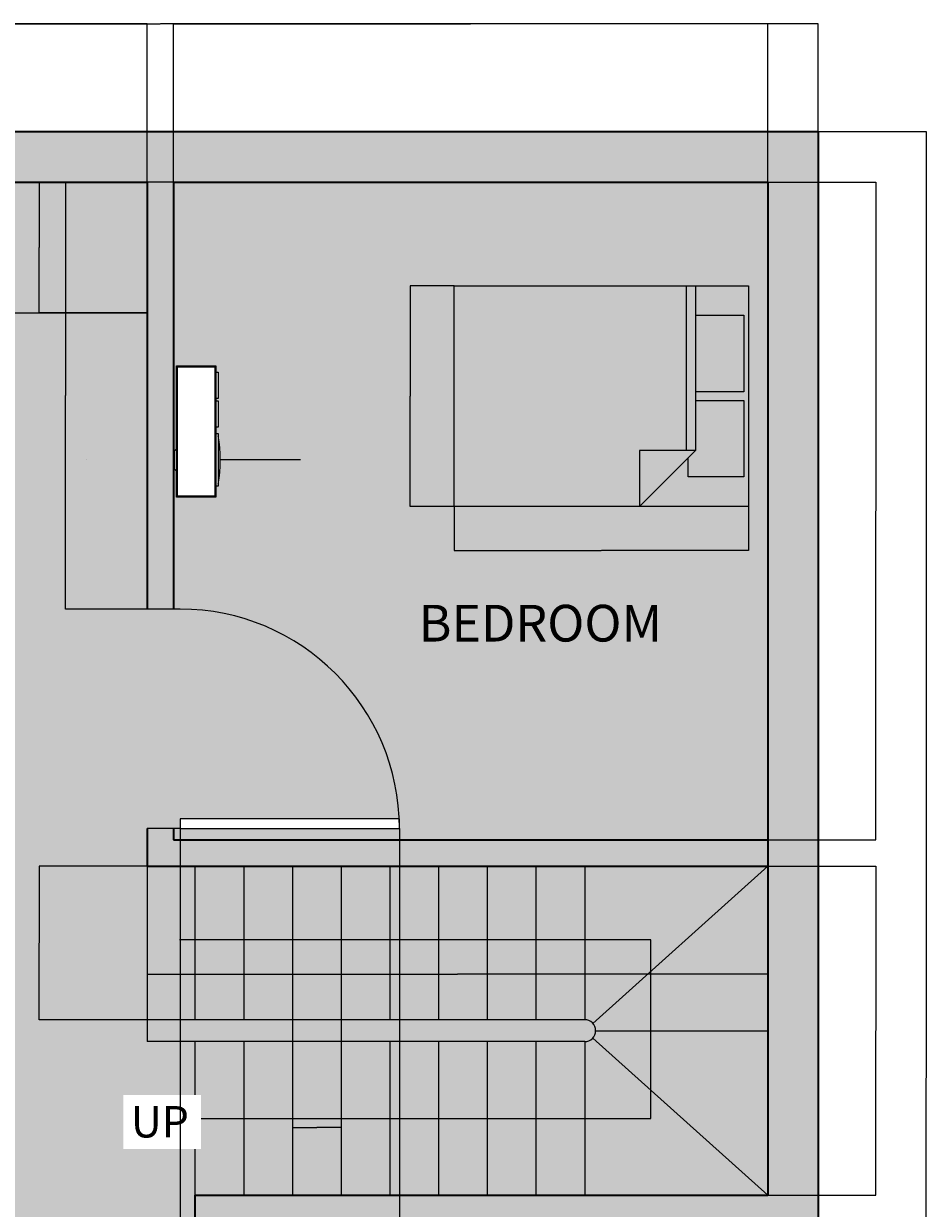
# Model space of a CAD drawing. Units: millimetres. Extents: x 1166 to 16630, y -7192 to 2820.
# Tile 6 of 8: x 4103 to 8218, y -2583 to 2820. Entities that reach past the tile are written whole.
import ezdxf

# ---------------------------------------------------------------- set-up
doc = ezdxf.new("R2010")
doc.units = ezdxf.units.MM
for name, color, linetype, lineweight in [('A-ANNO-DIMS', 2, 'Continuous', 18), ('A-ANNO-SYMB', 7, 'Continuous', 18), ('A-AREA-IDEN', 7, 'Continuous', 18), ('A-DOOR', 4, 'Continuous', 25), ('A-FLOR-CASE', 8, 'Continuous', 18), ('A-FLOR-STRS', 7, 'Continuous', 18), ('A-FURN', 8, 'Continuous', 18), ('A-WALL', 7, 'Continuous', 35)]:
    doc.layers.add(name, color=color, linetype=linetype, lineweight=lineweight)
for name, color, linetype, lineweight, true_color in [('A-FLOR-CASE-PATT', 9, 'Continuous', 13, 0xc7c8ca), ('A-FLOR-FNSH-PATT', 254, 'Continuous', 13, 0xfeeab9), ('A-FURN-PATT', 254, 'Continuous', 13, 0xd7c8d7), ('A-WALL-PATT', 254, 'Continuous', 13, 0xcecce6)]:
    doc.layers.add(name, color=color, linetype=linetype, lineweight=lineweight, true_color=true_color)
doc.styles.get("Standard").update_dxf_attribs({"font": 'arial.ttf'})
doc.dimstyles.get("Standard").update_dxf_attribs({"dimtxt": 0.18, "dimasz": 0.18, "dimexe": 0.18, "dimexo": 0.0625, "dimgap": 0.09, "dimtad": 0, "dimtih": 1, "dimtoh": 1, "dimdec": 4, "dimzin": 0, "dimdsep": 46, "dimtxsty": 'Standard', "dimcen": 0.09, "dimadec": 0, "dimazin": 0, "dimtfac": 1, "dimtdec": 4, "dimtofl": 0, "dimtmove": 0, "dimatfit": 3, "dimfxl": 1, "dimtolj": 1, "dimtzin": 0, "dimarcsym": 0})

# ---------------------------------------------------------------- blocks, each defined once
blk = doc.blocks.new('*U2')
for p, q in [((0, 0), (0, 6)), ((40, 0), (40, 6))]:
    blk.add_line(p, q)
blk.add_lwpolyline([(0, 0), (0, -40), (1.75, -40), (1.75, 0)], close=True)
blk.add_arc((0, 0), 40, 270, 0)
blk = doc.blocks.new('Bed - Queen')
for p, q in [((0, -80.00003), (0, 0)), ((0, 0), (59.99999, 0)), ((59.99999, 0), (59.99999, -80.00003)), ((7.99999, -1.2), (28.79998, -1.2)), ((7.99999, -14.4), (7.99999, -1.2)), ((28.79998, -1.2), (28.79998, -14.4)), ((31.19999, -1.2), (51.99999, -1.2)), ((31.19999, -14.4), (31.19999, -1.2)), ((51.99999, -1.2), (51.99999, -16.4)), ((0, -14.4), (44.8, -14.4)), ((59.99999, -29.6), (44.8, -14.4)), ((44.8, -14.4), (44.8, -29.6)), ((44.8, -16.8), (0, -16.8)), ((51.99999, -16.4), (46.79936, -16.4)), ((44.8, -29.6), (59.99999, -29.6)), ((59.99999, -80.00003), (0, -80.00003))]:
    blk.add_line(p, q)
blk = doc.blocks.new('Entertainment Center')
for p, q in [((-4, 0), (-5, -1)), ((4, 0), (-4, 0)), ((5, -1), (4, 0)), ((-17, -19), (-17, -1)), ((-17, -1), (43, -1)), ((-16.5, -18.5), (-16.5, -1.5)), ((-16.5, -1.5), (42.5, -1.5)), ((42.5, -1.5), (42.5, -18.5)), ((43, -1), (43, -19)), ((43, -19), (-17, -19)), ((42.5, -18.5), (-16.5, -18.5)), ((-12, -20), (-12, -19)), ((12, -20), (-12, -20)), ((12, -19), (12, -20)), ((15, -20), (15, -19)), ((27, -20), (15, -20)), ((27, -19), (27, -20)), ((28, -20), (28, -19)), ((40, -20), (28, -20)), ((40, -19), (40, -20))]:
    blk.add_line(p, q)
blk.add_arc((0, 40), 61, 259.6111, 280.3889)
blk = doc.blocks.new('*D13')
at = {"layer": 'A-ANNO-DIMS', "color": 0, "lineweight": -2, "transparency": 16777216}
for p, q in [((6066.1, 618.4), (6066.1, 417.1)), ((7407.1, 618.4), (7407.1, 417.1)), ((6066.3, 417.3), (6735.5, 417.3)), ((7406.9, 417.3), (6737.7, 417.3))]:
    blk.add_line(p, q, dxfattribs=at)
at = {"layer": 'A-ANNO-DIMS', "color": 0, "transparency": 16777216}
for points in [[(6066.3, 417.3), (6066.3, 417.2), (6066.1, 417.3)], [(7406.9, 417.3), (7406.9, 417.2), (7407.1, 417.3)]]:
    blk.add_solid(points, dxfattribs=at)
at = {"layer": 'Defpoints', "color": 0, "transparency": 16777216}
for p in [(6066.1, 618.4), (7407.1, 618.4), (7407.1, 417.3)]:
    blk.add_point(p, dxfattribs=at)
at = {"layer": 'A-ANNO-DIMS', "color": 0, "transparency": 16777216, "insert": (6736.6, 417.3), "char_height": 0.18, "attachment_point": 5}
blk.add_mtext('\\A1;QUEEN BED 1341', dxfattribs=at)
blk = doc.blocks.new('*D14')
at = {"layer": 'A-ANNO-DIMS', "color": 0, "lineweight": -2, "transparency": 16777216}
for p, q in [((6066, 1624.2), (5864.7, 1624.2)), ((5864.9, 1624), (5864.9, 1121.5)), ((5864.9, 618.6), (5864.9, 1121.1)), ((6066, 618.4), (5864.7, 618.4))]:
    blk.add_line(p, q, dxfattribs=at)
at = {"layer": 'A-ANNO-DIMS', "color": 0, "transparency": 16777216}
for points in [[(5864.9, 1624), (5865, 1624), (5864.9, 1624.2)], [(5864.9, 618.6), (5865, 618.6), (5864.9, 618.4)]]:
    blk.add_solid(points, dxfattribs=at)
at = {"layer": 'Defpoints', "color": 0, "transparency": 16777216}
for p in [(6066.1, 1624.2), (5864.9, 618.4), (6066.1, 618.4)]:
    blk.add_point(p, dxfattribs=at)
at = {"layer": 'A-ANNO-DIMS', "color": 0, "transparency": 16777216, "insert": (5864.9, 1121.3), "char_height": 0.18, "attachment_point": 5}
blk.add_mtext('\\A1;1006', dxfattribs=at)
blk = doc.blocks.new('*D23')
at = {"layer": 'A-ANNO-DIMS', "color": 0, "lineweight": -2, "transparency": 16777216}
for p, q in [((1725.9, 2327.5), (1725.9, 2819.6)), ((1726.1, 2819.5), (4725.6, 2819.5)), ((7725.8, 2819.5), (4726.3, 2819.5)), ((7725.9, 2327.5), (7725.9, 2819.6))]:
    blk.add_line(p, q, dxfattribs=at)
at = {"layer": 'A-ANNO-DIMS', "color": 0, "transparency": 16777216}
for points in [[(1726.1, 2819.5), (1726.1, 2819.4), (1725.9, 2819.5)], [(7725.8, 2819.5), (7725.8, 2819.4), (7725.9, 2819.5)]]:
    blk.add_solid(points, dxfattribs=at)
at = {"layer": 'Defpoints', "color": 0, "transparency": 16777216}
for p in [(7725.9, 2819.5), (1725.9, 2327.5), (7725.9, 2327.5)]:
    blk.add_point(p, dxfattribs=at)
at = {"layer": 'A-ANNO-DIMS', "color": 0, "transparency": 16777216, "insert": (4725.9, 2819.5), "char_height": 0.18, "attachment_point": 5}
blk.add_mtext('\\A1;6000', dxfattribs=at)
blk = doc.blocks.new('*D24')
at = {"layer": 'A-ANNO-DIMS', "color": 0, "lineweight": -2, "transparency": 16777216}
for p, q in [((7726, 2327.5), (8218.1, 2327.5)), ((8217.9, 2327.3), (8217.9, -1988.2)), ((8217.9, -6304), (8217.9, -1988.5)), ((7726, -6304.1), (8218.1, -6304.1))]:
    blk.add_line(p, q, dxfattribs=at)
at = {"layer": 'A-ANNO-DIMS', "color": 0, "transparency": 16777216}
for points in [[(8217.9, 2327.3), (8218, 2327.3), (8217.9, 2327.5)], [(8217.9, -6304), (8218, -6304), (8217.9, -6304.1)]]:
    blk.add_solid(points, dxfattribs=at)
at = {"layer": 'Defpoints', "color": 0, "transparency": 16777216}
for p in [(7725.9, 2327.5), (7725.9, -6304.1), (8217.9, -6304.1)]:
    blk.add_point(p, dxfattribs=at)
at = {"layer": 'A-ANNO-DIMS', "color": 0, "transparency": 16777216, "insert": (8217.9, -1988.3), "char_height": 0.18, "attachment_point": 5}
blk.add_mtext('\\A1;8632', dxfattribs=at)
blk = doc.blocks.new('*D25')
at = {"layer": 'A-ANNO-DIMS', "color": 0, "lineweight": -2, "transparency": 16777216}
for p, q in [((1955.939441, 2097.524735), (1955.939441, 2819.642235)), ((1956.119441, 2819.462235), (3310.579441, 2819.462235)), ((4665.759441, 2819.462235), (3311.299441, 2819.462235)), ((4665.939441, 2097.524735), (4665.939441, 2819.642235))]:
    blk.add_line(p, q, dxfattribs=at)
at = {"layer": 'A-ANNO-DIMS', "color": 0, "transparency": 16777216}
for points in [[(1956.119441, 2819.492235), (1956.119441, 2819.432235), (1955.939441, 2819.462235)], [(4665.759441, 2819.492235), (4665.759441, 2819.432235), (4665.939441, 2819.462235)]]:
    blk.add_solid(points, dxfattribs=at)
at = {"layer": 'Defpoints', "color": 0, "transparency": 16777216}
for p in [(4665.939441, 2819.462235), (1955.939441, 2097.462235), (4665.939441, 2097.462235)]:
    blk.add_point(p, dxfattribs=at)
at = {"layer": 'A-ANNO-DIMS', "color": 0, "transparency": 16777216, "insert": (3310.939441, 2819.462235), "char_height": 0.18, "attachment_point": 5}
blk.add_mtext('\\A1;2710', dxfattribs=at)
blk = doc.blocks.new('*D26')
at = {"layer": 'A-ANNO-DIMS', "color": 0, "lineweight": -2, "transparency": 16777216}
for p, q in [((4785.939441, 2097.524735), (4785.939441, 2819.642235)), ((4786.119441, 2819.462235), (6140.579441, 2819.462235)), ((7495.759441, 2819.462235), (6141.299441, 2819.462235)), ((7495.939441, 2097.524735), (7495.939441, 2819.642235))]:
    blk.add_line(p, q, dxfattribs=at)
at = {"layer": 'A-ANNO-DIMS', "color": 0, "transparency": 16777216}
for points in [[(4786.119441, 2819.492235), (4786.119441, 2819.432235), (4785.939441, 2819.462235)], [(7495.759441, 2819.492235), (7495.759441, 2819.432235), (7495.939441, 2819.462235)]]:
    blk.add_solid(points, dxfattribs=at)
at = {"layer": 'Defpoints', "color": 0, "transparency": 16777216}
for p in [(7495.939441, 2819.462235), (4785.939441, 2097.462235), (7495.939441, 2097.462235)]:
    blk.add_point(p, dxfattribs=at)
at = {"layer": 'A-ANNO-DIMS', "color": 0, "transparency": 16777216, "insert": (6140.939441, 2819.462235), "char_height": 0.18, "attachment_point": 5}
blk.add_mtext('\\A1;2710', dxfattribs=at)
blk = doc.blocks.new('*D33')
at = {"layer": 'A-ANNO-DIMS', "color": 0, "lineweight": -2, "transparency": 16777216}
for p, q in [((7496, 2097.5), (7988.1, 2097.5)), ((7987.9, 2097.3), (7987.9, 597.6)), ((7987.9, -902.4), (7987.9, 597.3)), ((7496, -902.5), (7988.1, -902.5))]:
    blk.add_line(p, q, dxfattribs=at)
at = {"layer": 'A-ANNO-DIMS', "color": 0, "transparency": 16777216}
for points in [[(7987.9, 2097.3), (7988, 2097.3), (7987.9, 2097.5)], [(7987.9, -902.4), (7988, -902.4), (7987.9, -902.5)]]:
    blk.add_solid(points, dxfattribs=at)
at = {"layer": 'Defpoints', "color": 0, "transparency": 16777216}
for p in [(7495.9, 2097.5), (7495.9, -902.5), (7987.9, -902.5)]:
    blk.add_point(p, dxfattribs=at)
at = {"layer": 'A-ANNO-DIMS', "color": 0, "transparency": 16777216, "insert": (7987.9, 597.5), "char_height": 0.18, "attachment_point": 5}
blk.add_mtext('\\A1;3000', dxfattribs=at)
blk = doc.blocks.new('*D34')
at = {"layer": 'A-ANNO-DIMS', "color": 0, "lineweight": -2, "transparency": 16777216}
for p, q in [((7496, -1022.5), (7988.1, -1022.5)), ((7987.9, -1022.7), (7987.9, -1772.4)), ((7987.9, -2522.4), (7987.9, -1772.7)), ((7496, -2522.5), (7988.1, -2522.5))]:
    blk.add_line(p, q, dxfattribs=at)
at = {"layer": 'A-ANNO-DIMS', "color": 0, "transparency": 16777216}
for points in [[(7987.9, -1022.7), (7988, -1022.7), (7987.9, -1022.5)], [(7987.9, -2522.4), (7988, -2522.4), (7987.9, -2522.5)]]:
    blk.add_solid(points, dxfattribs=at)
at = {"layer": 'Defpoints', "color": 0, "transparency": 16777216}
for p in [(7495.9, -1022.5), (7495.9, -2522.5), (7987.9, -2522.5)]:
    blk.add_point(p, dxfattribs=at)
at = {"layer": 'A-ANNO-DIMS', "color": 0, "transparency": 16777216, "insert": (7987.9, -1772.5), "char_height": 0.18, "attachment_point": 5}
blk.add_mtext('\\A1;1500', dxfattribs=at)
blk = doc.blocks.new('*D36')
at = {"layer": 'A-ANNO-DIMS', "color": 0, "lineweight": -2, "transparency": 16777216}
for p, q in [((4815.9, -849.9), (4815.9, -7065.6)), ((5815.9, -849.9), (5815.9, -7065.6)), ((4816.1, -7065.4), (5315.6, -7065.4)), ((5815.8, -7065.4), (5316.3, -7065.4))]:
    blk.add_line(p, q, dxfattribs=at)
at = {"layer": 'A-ANNO-DIMS', "color": 0, "transparency": 16777216}
for points in [[(4816.1, -7065.4), (4816.1, -7065.5), (4815.9, -7065.4)], [(5815.8, -7065.4), (5815.8, -7065.5), (5815.9, -7065.4)]]:
    blk.add_solid(points, dxfattribs=at)
at = {"layer": 'Defpoints', "color": 0, "transparency": 16777216}
for p in [(4815.9, -849.8), (5815.9, -849.8), (5815.9, -7065.4)]:
    blk.add_point(p, dxfattribs=at)
at = {"layer": 'A-ANNO-DIMS', "color": 0, "transparency": 16777216, "insert": (5315.9, -7065.4), "char_height": 0.18, "attachment_point": 5}
blk.add_mtext('\\A1;1000', dxfattribs=at)
blk = doc.blocks.new('*D40')
at = {"layer": 'A-ANNO-DIMS', "color": 0, "lineweight": -2, "transparency": 16777216}
for p, q in [((4665.9, 2097.5), (4173.8, 2097.5)), ((4173.9, 2097.3), (4173.9, 1799.3)), ((4173.9, 1500.9), (4173.9, 1798.9)), ((4665.9, 1500.7), (4173.8, 1500.7))]:
    blk.add_line(p, q, dxfattribs=at)
at = {"layer": 'A-ANNO-DIMS', "color": 0, "transparency": 16777216}
for points in [[(4173.9, 2097.3), (4174, 2097.3), (4173.9, 2097.5)], [(4173.9, 1500.9), (4174, 1500.9), (4173.9, 1500.7)]]:
    blk.add_solid(points, dxfattribs=at)
at = {"layer": 'Defpoints', "color": 0, "transparency": 16777216}
for p in [(4173.9, 2097.5), (4665.9, 2097.5), (4665.9, 1500.7)]:
    blk.add_point(p, dxfattribs=at)
at = {"layer": 'A-ANNO-DIMS', "color": 0, "transparency": 16777216, "insert": (4173.9, 1799.1), "char_height": 0.18, "attachment_point": 5}
blk.add_mtext('\\A1;596.8', dxfattribs=at)
blk = doc.blocks.new('*D42')
at = {"layer": 'A-ANNO-DIMS', "color": 0, "lineweight": -2, "transparency": 16777216}
for p, q in [((4785.9, 2097.5), (4293.8, 2097.5)), ((4293.9, 2097.3), (4293.9, 1124)), ((4293.9, 150.4), (4293.9, 1123.6)), ((4785.9, 150.2), (4293.8, 150.2))]:
    blk.add_line(p, q, dxfattribs=at)
at = {"layer": 'A-ANNO-DIMS', "color": 0, "transparency": 16777216}
for points in [[(4293.9, 2097.3), (4294, 2097.3), (4293.9, 2097.5)], [(4293.9, 150.4), (4294, 150.4), (4293.9, 150.2)]]:
    blk.add_solid(points, dxfattribs=at)
at = {"layer": 'Defpoints', "color": 0, "transparency": 16777216}
for p in [(4293.9, 2097.5), (4785.9, 2097.5), (4785.9, 150.2)]:
    blk.add_point(p, dxfattribs=at)
at = {"layer": 'A-ANNO-DIMS', "color": 0, "transparency": 16777216, "insert": (4293.9, 1123.8), "char_height": 0.18, "attachment_point": 5}
blk.add_mtext('\\A1;1947.3', dxfattribs=at)
blk = doc.blocks.new('*D44')
at = {"layer": 'A-ANNO-DIMS', "color": 0, "lineweight": -2, "transparency": 16777216}
for p, q in [((4665.9, -1022.5), (4173.8, -1022.5)), ((4173.9, -1022.7), (4173.9, -1372.4)), ((4173.9, -1722.4), (4173.9, -1372.7)), ((4665.9, -1722.5), (4173.8, -1722.5))]:
    blk.add_line(p, q, dxfattribs=at)
at = {"layer": 'A-ANNO-DIMS', "color": 0, "transparency": 16777216}
for points in [[(4173.9, -1022.7), (4174, -1022.7), (4173.9, -1022.5)], [(4173.9, -1722.4), (4174, -1722.4), (4173.9, -1722.5)]]:
    blk.add_solid(points, dxfattribs=at)
at = {"layer": 'Defpoints', "color": 0, "transparency": 16777216}
for p in [(4173.9, -1022.5), (4665.9, -1022.5), (4665.9, -1722.5)]:
    blk.add_point(p, dxfattribs=at)
at = {"layer": 'A-ANNO-DIMS', "color": 0, "transparency": 16777216, "insert": (4173.9, -1372.5), "char_height": 0.18, "attachment_point": 5}
blk.add_mtext('\\A1;700', dxfattribs=at)
blk = doc.blocks.new('*D45')
at = {"layer": 'A-ANNO-DIMS', "color": 0, "lineweight": -2, "transparency": 16777216}
for p, q in [((5328.2, -1722.6), (5328.2, -2214.7)), ((5550.3, -1722.6), (5550.3, -2214.7)), ((5328.4, -2214.5), (5438.9, -2214.5)), ((5550.1, -2214.5), (5439.6, -2214.5))]:
    blk.add_line(p, q, dxfattribs=at)
at = {"layer": 'A-ANNO-DIMS', "color": 0, "transparency": 16777216}
for points in [[(5328.4, -2214.5), (5328.4, -2214.6), (5328.2, -2214.5)], [(5550.1, -2214.5), (5550.1, -2214.6), (5550.3, -2214.5)]]:
    blk.add_solid(points, dxfattribs=at)
at = {"layer": 'Defpoints', "color": 0, "transparency": 16777216}
for p in [(5328.2, -1722.5), (5550.3, -1722.5), (5328.2, -2214.5)]:
    blk.add_point(p, dxfattribs=at)
at = {"layer": 'A-ANNO-DIMS', "color": 0, "transparency": 16777216, "insert": (5439.2, -2214.5), "char_height": 0.18, "attachment_point": 5}
blk.add_mtext('\\A1;222.1', dxfattribs=at)
blk = doc.blocks.new('*D46')
at = {"layer": 'A-ANNO-DIMS', "color": 0, "lineweight": -2, "transparency": 16777216}
for p, q in [((4665.939441, -1022.600265), (4665.939441, -1514.717765)), ((7495.939441, -1022.600265), (7495.939441, -1514.717765)), ((4666.119441, -1514.537765), (6080.579441, -1514.537765)), ((7495.759441, -1514.537765), (6081.299441, -1514.537765))]:
    blk.add_line(p, q, dxfattribs=at)
at = {"layer": 'A-ANNO-DIMS', "color": 0, "transparency": 16777216}
for points in [[(4666.119441, -1514.507765), (4666.119441, -1514.567765), (4665.939441, -1514.537765)], [(7495.759441, -1514.507765), (7495.759441, -1514.567765), (7495.939441, -1514.537765)]]:
    blk.add_solid(points, dxfattribs=at)
at = {"layer": 'Defpoints', "color": 0, "transparency": 16777216}
for p in [(4665.939441, -1022.537765), (7495.939441, -1022.537765), (4665.939441, -1514.537765)]:
    blk.add_point(p, dxfattribs=at)
at = {"layer": 'A-ANNO-DIMS', "color": 0, "transparency": 16777216, "insert": (6080.939441, -1514.537765), "char_height": 0.18, "attachment_point": 5}
blk.add_mtext('\\A1;2830', dxfattribs=at)
blk = doc.blocks.new('*D71')
at = {"layer": 'A-ANNO-DIMS', "color": 0, "lineweight": -2, "transparency": 16777216}
for p, q in [((4389.3, 830.2), (4389.5, 830.2)), ((4389.4, 830.1), (4389.4, 830.2)), ((5365.1, 830.2), (4999.4, 830.2))]:
    blk.add_line(p, q, dxfattribs=at)
at = {"layer": 'A-ANNO-DIMS', "color": 0, "transparency": 16777216}
blk.add_solid([(4999.4, 830.2), (4999.4, 830.1), (4999.2, 830.2)], dxfattribs=at)
at = {"layer": 'Defpoints', "color": 0, "transparency": 16777216}
for p in [(4389.4, 830.2), (4999.2, 830.2)]:
    blk.add_point(p, dxfattribs=at)
at = {"layer": 'A-ANNO-DIMS', "color": 0, "transparency": 16777216, "insert": (5365.5, 830.2), "char_height": 0.18, "attachment_point": 5}
blk.add_mtext('\\A1;R609.8', dxfattribs=at)

msp = doc.modelspace()

# ---------------------------------------------------------------- hatches: boundary and pattern name
at = {"layer": 'A-FLOR-CASE-PATT'}
h = msp.add_hatch(color=256, dxfattribs=at)
h.dxf.hatch_style = 1
h.paths.add_polyline_path([(2460.545, 1500.697), (4665.939, 1500.697), (4665.939, 2097.462), (1955.939, 2097.462), (1955.939, -402.538), (2460.545, -402.538)])
at = {"layer": 'A-FLOR-FNSH-PATT', "transparency": 33554523}
h = msp.add_hatch(color=256, dxfattribs=at)
h.dxf.hatch_style = 1
h.paths.add_polyline_path([(7725.939, 2327.462), (1725.939, 2327.462), (1725.939, -5672.538), (5309.615, -5672.538), (5309.615, -2642.538), (5189.615, -2642.538), (5189.615, -5442.538), (1955.939, -5442.538), (1955.939, 2097.462), (4665.939, 2097.462), (4665.939, 150.2), (4815.939, 150.2, -0.40145271), (5814.982, -806.05), (5815.939, -806.05), (5815.939, -849.8), (4815.939, -849.8), (4785.939, -849.8), (4785.939, -902.538), (7495.939, -902.538), (7495.939, -2522.538), (4884.014, -2522.538), (4884.014, -2642.538), (7725.939, -2642.538)], flags=17)
h.paths.add_polyline_path([(6066.077, 618.421), (6066.077, 1624.186), (7407.098, 1624.186), (7407.098, 618.421)], flags=16)
h.paths.add_polyline_path([(4979.212, 660.219), (4799.278, 660.219), (4799.278, 780.174), (4789.282, 790.171), (4789.282, 870.141), (4799.278, 880.137), (4799.278, 1259.997), (4979.212, 1259.997), (4979.212, 1230.008), (4989.208, 1230.008), (4989.208, 1110.052), (4979.212, 1110.052), (4979.212, 1100.056), (4989.208, 1100.056), (4989.208, 980.1), (4979.212, 980.1), (4979.212, 950.111), (4989.208, 950.111), (4989.208, 940.115, -0.09090909), (4989.208, 720.196), (4989.208, 710.2), (4979.212, 710.2)], flags=16)
h.paths.add_polyline_path([(4974.214, 665.217), (4804.276, 665.217), (4804.276, 1254.999), (4974.214, 1254.999)], flags=0)
h.paths.add_polyline_path([(6910.92, 618.421), (6910.92, 873.215), (7165.714, 873.215), (7165.714, 1490.084), (7386.983, 1490.084), (7386.983, 1141.419), (7165.714, 1141.419), (7165.714, 1101.188), (7386.983, 1101.188), (7386.983, 752.523), (7132.189, 752.523), (7132.189, 839.689)], flags=16)
h.paths.add_polyline_path([(4815.939, 150.2), (4665.939, 150.2), (4665.939, 1500.697), (2460.545, 1500.697), (2460.545, -402.538), (3575.939, -402.538), (3575.939, -1706.64), (3463.439, -1706.64, 0.40145271), (2714.158, -2423.828), (3463.439, -2423.828), (3463.439, -2456.64), (3455.939, -2522.538), (3455.939, -2456.64), (2713.439, -2456.64), (2713.439, -2423.828), (2714.158, -2423.828, -0.39855266), (3455.939, -1706.678), (3455.939, -1706.64), (3575.939, -1706.64), (3575.939, -402.538), (2460.545, -402.538), (2460.545, 1500.697), (4665.939, 1500.697), (4665.939, 150.2), (4785.939, 150.2), (4785.939, 2097.462), (7495.939, 2097.462), (7495.939, -2522.538), (4884.014, -2522.538), (4884.014, -2642.538), (7725.939, -2642.538), (7725.939, 2327.462), (1725.939, 2327.462), (1725.939, -5672.538), (5309.615, -5672.538), (5309.615, -2642.538), (4884.014, -2642.538), (4884.014, -2522.538), (4884.014, -1822.538), (4665.939, -1822.538), (4665.939, -1722.538), (4665.939, -1022.538), (4665.939, -849.8), (4815.939, -849.8), (4815.939, -806.05), (5814.982, -806.05, 0.40145271)])
h.paths.add_polyline_path([(1955.939, -4323.626), (1965.936, -4313.63), (1965.936, -3933.77), (2145.869, -3933.77), (2145.869, -3963.759), (2155.866, -3963.759), (2155.866, -4083.715), (2145.869, -4083.715), (2145.869, -4093.711), (2155.866, -4093.711), (2155.866, -4213.667), (2145.869, -4213.667), (2145.869, -4243.656), (2155.866, -4243.656), (2155.866, -4253.652, -0.09090909), (2155.866, -4473.571), (2155.866, -4483.567), (2145.869, -4483.567), (2145.869, -4533.549), (1965.936, -4533.549), (1965.936, -4413.593), (1955.939, -4403.597)], flags=16)
h.paths.add_polyline_path([(3017.672, -1268.685), (3017.672, -1558.932), (2092.538, -1558.932), (2092.538, -1268.685)], flags=16)
h.paths.add_polyline_path([(2768.799, -687.028), (2664.904, -687.028), (2696.871, -782.93, -0.50132349), (2617.667, -1084.405, -0.13289091), (2584.271, -1084.405, -0.50131678), (2505.065, -782.933), (2537.033, -687.028), (2489.082, -687.028), (2489.082, -711.004), (2441.13, -711.004), (2441.13, -687.028), (2433.138, -687.028), (2433.138, -559.158), (2768.799, -559.158)], flags=16)
h.paths.add_polyline_path([(2752.815, -655.061, -0.41421356), (2740.827, -671.045), (2465.106, -671.045, -0.41421356), (2449.122, -659.057), (2449.122, -591.126, -0.41421356), (2461.11, -575.142), (2736.831, -575.142, -0.41421356), (2752.815, -587.13)], flags=0)
h.paths.add_polyline_path([(2627.247, -1063.016, -0.21500378), (2574.691, -1063.016, -0.48007965), (2537.034, -782.931), (2664.904, -782.931, -0.4800795)], flags=0)
h.paths.add_polyline_path([(4505.634, -3647.875), (4977.863, -3647.875, -0.19047621), (4977.864, -5173.541), (4505.634, -5173.541), (4505.634, -5064.565), (4533.929, -5064.565), (4533.929, -3756.851), (4505.634, -3756.851)], flags=16)
h.paths.add_polyline_path([(4880.114, -4192.756), (5003.372, -4192.756, -0.04962821), (5003.372, -4628.66), (4880.114, -4628.66)], flags=0)
h.paths.add_polyline_path([(2140.871, -3938.769), (2140.871, -4528.551), (1970.934, -4528.551), (1970.934, -3938.769)], flags=0)
h.paths.add_polyline_path([(7495.939, -1022.538), (6660.699, -1022.538), (6660.699, -1722.538, -0.21291191), (6697.901, -1739.132)], flags=16)
h.paths.add_polyline_path([(7495.939, -1022.538), (6697.901, -1739.132, -0.18498743), (6710.699, -1772.538), (7495.939, -1772.538)], flags=16)
h.paths.add_polyline_path([(7495.939, -1772.538), (6710.699, -1772.538, -0.18498743), (6697.901, -1805.944), (7495.939, -2522.538)], flags=16)
h.paths.add_polyline_path([(6697.901, -1805.944, -0.21291191), (6660.699, -1822.538), (6660.699, -2522.538), (7495.939, -2522.538)], flags=16)
h.paths.add_polyline_path([(6660.699, -1822.538), (6438.613, -1822.538), (6438.613, -2522.538), (6660.699, -2522.538)], flags=16)
h.paths.add_polyline_path([(6438.613, -1822.538), (6216.528, -1822.538), (6216.528, -2522.538), (6438.613, -2522.538)], flags=16)
h.paths.add_polyline_path([(6216.528, -1822.538), (5994.442, -1822.538), (5994.442, -2522.538), (6216.528, -2522.538)], flags=16)
h.paths.add_polyline_path([(5994.442, -1822.538), (5772.357, -1822.538), (5772.357, -2522.538), (5994.442, -2522.538)], flags=16)
h.paths.add_polyline_path([(5550.271, -1822.538), (5328.185, -1822.538), (5328.185, -2522.538), (5550.271, -2522.538)], flags=16)
h.paths.add_polyline_path([(5328.185, -1822.538), (5106.1, -1822.538), (5106.1, -2522.538), (5328.185, -2522.538)], flags=16)
h.paths.add_polyline_path([(5106.1, -1822.538), (4884.014, -1822.538), (4884.014, -2522.538), (5106.1, -2522.538)], flags=16)
h.paths.add_polyline_path([(4884.014, -1022.538), (4665.939, -1022.538), (4665.939, -1722.538), (4884.014, -1722.538)], flags=16)
h.paths.add_polyline_path([(5106.1, -1022.538), (4884.014, -1022.538), (4884.014, -1722.538), (5106.1, -1722.538)], flags=16)
h.paths.add_polyline_path([(5550.271, -1022.538), (5328.185, -1022.538), (5328.185, -1722.538), (5550.271, -1722.538)], flags=16)
h.paths.add_polyline_path([(5328.185, -1022.538), (5106.1, -1022.538), (5106.1, -1722.538), (5328.185, -1722.538)], flags=16)
h.paths.add_polyline_path([(5772.357, -1022.538), (5550.271, -1022.538), (5550.271, -1722.538), (5772.357, -1722.538)], flags=16)
h.paths.add_polyline_path([(5994.442, -1022.538), (5772.357, -1022.538), (5772.357, -1722.538), (5994.442, -1722.538)], flags=16)
h.paths.add_polyline_path([(6216.528, -1022.538), (5994.442, -1022.538), (5994.442, -1722.538), (6216.528, -1722.538)], flags=16)
h.paths.add_polyline_path([(6660.699, -1022.538), (6438.613, -1022.538), (6438.613, -1722.538), (6660.699, -1722.538)], flags=16)
h.paths.add_polyline_path([(6438.613, -1022.538), (6216.528, -1022.538), (6216.528, -1722.538), (6438.613, -1722.538)], flags=16)
h.paths.add_polyline_path([(5772.357, -1822.538), (5550.271, -1822.538), (5550.271, -2522.538), (5772.357, -2522.538)], flags=16)
h.paths.add_polyline_path([(6660.699, -1722.538), (6438.613, -1722.538), (4665.939, -1722.538), (4665.939, -1822.538), (6660.699, -1822.538, 0.21291191), (6697.901, -1805.944, 0.64892437)], flags=16)
h.paths.add_polyline_path([(5860.25, -44.006), (7154.504, -44.006), (7154.504, 215.689), (5860.25, 215.689)], flags=24)
h.paths.add_polyline_path([(2102.336, -1543.656), (3007.075, -1543.656), (3007.075, -1283.961), (2102.336, -1283.961)], flags=8)
h.paths.add_polyline_path([(2887.503, -4248.68), (3740.372, -4248.68), (3740.372, -3989.156), (2887.503, -3989.156)], flags=24)
h.paths.add_polyline_path([(2999.436, 433.054), (4111.829, 433.054), (4111.829, 692.578), (2999.436, 692.578)], flags=24)
at = {"layer": 'A-FLOR-FNSH-PATT', "transparency": 33554590}
h = msp.add_hatch(color=256, dxfattribs=at)
h.dxf.hatch_style = 1
h.paths.add_polyline_path([(5309.615, -2642.538), (5309.615, -6304.141), (7725.939, -6304.141), (7725.939, -5672.538), (7725.939, -2642.538)])
edge = h.paths.add_edge_path(flags=16)
edge.add_ellipse((-448.972, -3645.43), major_axis=(-7430.723, 0), ratio=0.84230387, start_angle=182.1799503, end_angle=183.6504276, ccw=False)
edge.add_line((6974.174, -3362.862), (6984.716, -3362.862))
edge.add_ellipse((6982.281, -3380.397), major_axis=(-20.817, 0), ratio=0.84230387, start_angle=180, end_angle=270, ccw=False)
edge.add_line((7003.098, -3380.397), (7003.098, -3722.916))
edge.add_ellipse((6982.281, -3720.865), major_axis=(20.817, 0), ratio=0.84230387, start_angle=270, end_angle=360, ccw=False)
edge.add_ellipse((-142030.923, -3973.064), major_axis=(149013.204, 0), ratio=0.8423038695, start_angle=-0.38386678, end_angle=0.09022909, ccw=False)
edge.add_line((6977.567, -4971.397), (6984.47, -4971.397))
edge.add_ellipse((6982.281, -4988.932), major_axis=(20.817, 0), ratio=0.84230387, start_angle=0, end_angle=90, ccw=False)
edge.add_line((7003.098, -4988.932), (7003.098, -5331.243))
edge.add_ellipse((6982.281, -5329.4), major_axis=(-20.817, 0), ratio=0.84230387, start_angle=90, end_angle=180, ccw=False)
edge.add_line((6982.281, -5346.934), (6973.354, -5346.934))
edge.add_ellipse((-142030.923, -3973.064), major_axis=(149013.204, 0), ratio=0.8423038695, start_angle=-0.6186432, end_angle=-0.52827147, ccw=False)
edge.add_ellipse((6960.189, -5606.903), major_axis=(-31.226, 0), ratio=0.84230387, start_angle=179.371763, end_angle=248.464757, ccw=False)
edge.add_ellipse((-142041.332, -3973.064), major_axis=(-149045.372, 0), ratio=0.8423038661, start_angle=179.35344592, end_angle=179.3717628, ccw=False)
edge.add_ellipse((6916.87, -5654.054), major_axis=(-73.802, 0), ratio=0.84230387, start_angle=90, end_angle=179.353446, ccw=False)
edge.add_line((6916.87, -5716.218), (5995.23, -5716.218))
edge.add_ellipse((5995.23, -5654.054), major_axis=(73.802, 0), ratio=0.84230387, start_angle=180.646554, end_angle=270, ccw=False)
edge.add_ellipse((154953.432, -3973.064), major_axis=(-149045.372, 0), ratio=0.8423038697, start_angle=0.62823722, end_angle=0.6465541, ccw=False)
edge.add_ellipse((5951.911, -5606.903), major_axis=(31.226, 0), ratio=0.84230387, start_angle=111.535244, end_angle=180.628237, ccw=False)
edge.add_ellipse((154943.023, -3973.064), major_axis=(-149013.204, 0), ratio=0.8423038695, start_angle=0.52827147, end_angle=0.6465541, ccw=False)
edge.add_line((5938.746, -5346.934), (5927.384, -5346.934))
edge.add_ellipse((5929.819, -5329.4), major_axis=(20.817, 0), ratio=0.84230387, start_angle=180, end_angle=270, ccw=False)
edge.add_line((5909.002, -5329.4), (5909.002, -4986.881))
edge.add_ellipse((5929.819, -4988.932), major_axis=(-20.817, 0), ratio=0.84230387, start_angle=-90, end_angle=0, ccw=False)
edge.add_line((5929.819, -4971.397), (5934.533, -4971.397))
edge.add_ellipse((154943.023, -3973.064), major_axis=(-149013.204, 0), ratio=0.8423038695, start_angle=-0.09022909, end_angle=0.38386678, ccw=False)
edge.add_ellipse((5929.819, -3720.865), major_axis=(-20.817, 0), ratio=0.84230387, start_angle=0, end_angle=90, ccw=False)
edge.add_line((5909.002, -3720.865), (5909.002, -3378.346))
edge.add_ellipse((5929.819, -3380.397), major_axis=(20.817, 0), ratio=0.84230387, start_angle=90, end_angle=180, ccw=False)
edge.add_line((5929.819, -3362.862), (5937.926, -3362.862))
edge.add_ellipse((13361.072, -3645.43), major_axis=(7430.723, 0), ratio=0.84230387, start_angle=176.3495724, end_angle=177.8200497, ccw=False)
edge.add_ellipse((6843.239, -6808.261), major_axis=(4407.333, 0), ratio=0.84230387, start_angle=102.125966, end_angle=103.780529, ccw=False)
edge.add_ellipse((6843.239, -6711.831), major_axis=(4294.728, 0), ratio=0.84230387, start_angle=100.209539, end_angle=102.444627, ccw=False)
edge.add_ellipse((5718.978, -189.342), major_axis=(-3530.283, 0), ratio=0.84230387, start_angle=99.256566, end_angle=102.554933)
edge.add_line((6369.843, -3111.939), (6452.047, -3066.483))
edge.add_ellipse((6456.05, -3074.757), major_axis=(-10.409, 0), ratio=0.84230387, start_angle=270, end_angle=307.93313, ccw=False)
edge.add_ellipse((6456.05, -3074.757), major_axis=(-10.409, 0), ratio=0.84230387, start_angle=232.06687, end_angle=270, ccw=False)
edge.add_line((6461.762, -3067.428), (6542.257, -3111.939))
edge.add_ellipse((7193.122, -189.342), major_axis=(3530.283, 0), ratio=0.84230387, start_angle=257.445067, end_angle=260.743434)
edge.add_ellipse((6068.861, -6711.831), major_axis=(4294.728, 0), ratio=0.84230387, start_angle=77.555373, end_angle=79.790461, ccw=False)
edge.add_ellipse((6068.861, -6808.261), major_axis=(-4407.333, 0), ratio=0.84230387, start_angle=256.219471, end_angle=257.874034, ccw=False)
edge = h.paths.add_edge_path(flags=0)
edge.add_ellipse((5799.636, -3484.806), major_axis=(790.133, 0), ratio=0.84230387, start_angle=0, end_angle=29.43857, ccw=False)
edge.add_line((6589.77, -3484.806), (6589.77, -3517.866))
edge.add_line((6589.77, -3517.866), (6615.397, -3517.866))
edge.add_ellipse((6612.95, -3526.633), major_axis=(10.409, 0), ratio=0.84230387, start_angle=45.519789, end_angle=90, ccw=False)
edge.add_line((6619.584, -3519.877), (6697.577, -3574.216))
edge.add_line((6697.577, -3574.216), (6697.577, -3782.552))
edge.add_ellipse((6643.673, -3780.461), major_axis=(5.016, 89.187), ratio=0.60383358, start_angle=106.342592, end_angle=270.997986, ccw=False)
edge.add_line((6589.77, -3793.028), (6589.77, -3484.806))
edge.add_ellipse((5799.636, -3484.806), major_axis=(790.133, 0), ratio=0.84230387, start_angle=0, end_angle=29.43857)
edge.add_ellipse((7112.464, -3484.806), major_axis=(-790.133, 0), ratio=0.84230387, start_angle=-29.43857, end_angle=0)
edge.add_line((6322.33, -3484.806), (6322.33, -3793.028))
edge.add_ellipse((6268.427, -3780.461), major_axis=(-5.016, 89.187), ratio=0.60383358, start_angle=89.002014, end_angle=253.657408, ccw=False)
edge.add_line((6214.523, -3782.552), (6214.523, -3574.216))
edge.add_line((6214.523, -3574.216), (6294.401, -3518.564))
edge.add_ellipse((6299.15, -3526.633), major_axis=(10.409, 0), ratio=0.84230387, start_angle=90, end_angle=134.480211, ccw=False)
edge.add_line((6299.15, -3517.866), (6322.33, -3517.866))
edge.add_line((6322.33, -3517.866), (6322.33, -3484.806))
edge.add_ellipse((7112.464, -3484.806), major_axis=(-790.133, 0), ratio=0.84230387, start_angle=-29.43857, end_angle=0, ccw=False)
edge = h.paths.add_edge_path(flags=0)
edge.add_line((6899.672, -4051.113), (6868.937, -4281.474))
edge.add_ellipse((6495.43, -5170.363), major_axis=(1119.455, 0), ratio=0.84230387, start_angle=67.208085, end_angle=85.12993)
edge.add_line((6575.565, -4229.86), (6336.535, -4229.86))
edge.add_ellipse((6416.67, -5170.363), major_axis=(1119.455, 0), ratio=0.84230387, start_angle=94.87007, end_angle=112.791915)
edge.add_line((6043.163, -4281.474), (6012.428, -4051.113))
edge.add_ellipse((6380.264, -4969.144), major_axis=(1150.303, 0), ratio=0.84230387, start_angle=94.277421, end_angle=111.834954, ccw=False)
edge.add_line((6307.939, -4002.156), (6604.161, -4002.156))
edge.add_ellipse((6531.836, -4969.144), major_axis=(-1150.303, 0), ratio=0.84230387, start_angle=248.165046, end_angle=265.722579, ccw=False)
edge = h.paths.add_edge_path(flags=0)
edge.add_ellipse((-142030.923, -3973.064), major_axis=(-148992.387, 0), ratio=0.8423038695, start_angle=179.62223581, end_angle=179.94440569, ccw=False)
edge.add_line((6956.9, -4955.389), (6903.068, -4744.03))
edge.add_ellipse((-45118.924, -4413.46), major_axis=(52023.473, 0), ratio=0.84230387, start_angle=-0.3640763, end_angle=0.1208974)
edge.add_line((6904.386, -4303.688), (6961.365, -4117.632))
edge = h.paths.add_edge_path(flags=0)
edge.add_line((5950.735, -4117.632), (6007.714, -4303.688))
edge.add_ellipse((58031.024, -4413.46), major_axis=(-52023.473, 0), ratio=0.84230387, start_angle=-0.1208974, end_angle=0.3640763)
edge.add_line((6009.031, -4744.03), (5955.2, -4955.389))
edge.add_ellipse((154943.023, -3973.064), major_axis=(-148992.387, 0), ratio=0.8423038696, start_angle=0.05559431, end_angle=0.37776419, ccw=False)
edge = h.paths.add_edge_path(flags=0)
edge.add_line((6868.937, -5013.198), (6868.937, -5277.993))
edge.add_ellipse((6456.05, -3571.079), major_axis=(2068.116, 0), ratio=0.84230387, start_angle=256.401865, end_angle=283.598135, ccw=False)
edge.add_line((6043.163, -5277.993), (6043.163, -5013.198))
edge.add_ellipse((6456.05, -3306.285), major_axis=(2068.116, 0), ratio=0.84230387, start_angle=256.401865, end_angle=283.598135)
edge = h.paths.add_edge_path(flags=0)
edge.add_ellipse((6827.303, -5415.313), major_axis=(-41.634, 0), ratio=0.84230387, start_angle=180, end_angle=270, ccw=False)
edge.add_line((6868.937, -5415.313), (6868.937, -5689.123))
edge.add_line((6868.937, -5689.123), (6043.163, -5689.123))
edge.add_line((6043.163, -5689.123), (6043.163, -5415.313))
edge.add_ellipse((6084.797, -5415.313), major_axis=(-41.634, 0), ratio=0.84230387, start_angle=-90, end_angle=0, ccw=False)
edge.add_line((6084.797, -5380.245), (6827.303, -5380.245))
h.paths.add_polyline_path([(3455.939, -522.538), (1955.939, -522.538), (1955.939, -2522.538), (3455.939, -2522.538), (3455.939, -2456.64), (2713.439, -2456.64), (2713.439, -2423.828), (2714.158, -2423.828, -0.39855266), (3455.939, -1706.678)])
h.paths.add_polyline_path([(2617.667, -1084.405, -0.13289091), (2584.271, -1084.405, -0.50131678), (2505.065, -782.933), (2537.033, -687.028), (2489.082, -687.028), (2489.082, -711.004), (2441.13, -711.004), (2441.13, -695.02), (2473.098, -695.02), (2473.098, -687.028), (2433.138, -687.028), (2433.138, -559.158), (2768.799, -559.158), (2768.799, -687.028), (2664.904, -687.028), (2696.871, -782.93, -0.50132349)], flags=16)
h.paths.add_polyline_path([(2627.247, -1063.016, -0.21500378), (2574.691, -1063.016, -0.48007965), (2537.034, -782.931), (2664.904, -782.931, -0.4800795)], flags=0)
h.paths.add_polyline_path([(2736.831, -671.045), (2465.106, -671.045, -0.50000012), (2449.122, -655.061), (2449.122, -591.126, -0.50000012), (2465.106, -575.142), (2736.831, -575.142, -0.50000012), (2752.815, -591.126), (2752.815, -655.061, -0.50000012)], flags=0)
h.paths.add_polyline_path([(5931.782, -6111.826), (7070.31, -6111.826), (7070.31, -5852.302), (5931.782, -5852.302)], flags=24)
h.paths.add_polyline_path([(2102.336, -1543.656), (3007.075, -1543.656), (3007.075, -1283.961), (2102.336, -1283.961)], flags=24)
at = {"layer": 'A-FURN-PATT', "transparency": 33554615}
h = msp.add_hatch(color=256, dxfattribs=at)
h.dxf.hatch_style = 1
h.paths.add_polyline_path([(7125.484, 1624.186), (6066.077, 1624.186), (6066.077, 618.421), (6910.92, 618.421), (6910.92, 873.215), (7125.484, 873.215)])
at = {"layer": 'A-FURN-PATT'}
h = msp.add_hatch(color=256, dxfattribs=at)
h.dxf.hatch_style = 1
h.paths.add_polyline_path([(7165.714, 1624.186), (7125.484, 1624.186), (7125.484, 873.215), (7165.714, 873.215)], flags=17)
h.paths.add_polyline_path([(7407.098, 1624.186), (7165.714, 1624.186), (7165.714, 1490.084), (7386.983, 1490.084), (7386.983, 1141.419), (7165.714, 1141.419), (7165.714, 1101.188), (7386.983, 1101.188), (7386.983, 752.523), (7132.189, 752.523), (7132.189, 839.689), (6910.92, 618.421), (7407.098, 618.421)])
h.paths.add_polyline_path([(7165.714, 873.215), (6910.92, 873.215), (6910.92, 618.421)], flags=17)
at = {"layer": 'A-WALL-PATT'}
h = msp.add_hatch(color=256, dxfattribs=at)
h.dxf.hatch_style = 1
h.paths.add_polyline_path([(1955.939, 2097.462), (4665.939, 2097.462), (4665.939, 150.2), (4785.939, 150.2), (4785.939, 2097.462), (7495.939, 2097.462), (7495.939, -2522.538), (4884.014, -2522.538), (4884.014, -2642.538), (7725.939, -2642.538), (7725.939, 2327.462), (1725.939, 2327.462), (1725.939, -5672.538), (5309.615, -5672.538), (5309.615, -2642.538), (5189.615, -2642.538), (5189.615, -5442.538), (1955.939, -5442.538)])
h.paths.add_polyline_path([(7495.939, -902.538), (4785.939, -902.538), (4785.939, -849.8), (4665.939, -849.8), (4665.939, -1022.538), (7495.939, -1022.538)], flags=17)
h.paths.add_polyline_path([(3575.939, -402.538), (1955.939, -402.538), (1955.939, -522.538), (3455.939, -522.538), (3455.939, -1706.64), (3575.939, -1706.64)], flags=17)
h.paths.add_polyline_path([(3575.939, -2456.64), (3455.939, -2456.64), (3455.939, -2522.538), (1955.939, -2522.538), (1955.939, -2642.538), (3575.939, -2642.538)], flags=17)

# ---------------------------------------------------------------- linework, layer by layer
at = {"layer": 'A-ANNO-SYMB'}
for p, q in [((4884.014, -1358.888), (4813.503, -1358.888)), ((6962.098, -1358.888), (4884.014, -1358.888)), ((6962.098, -2172.538), (6962.098, -1358.888)), ((4884.014, -2172.538), (6962.098, -2172.538))]:
    msp.add_line(p, q, dxfattribs=at)
at = {"layer": 'A-FLOR-CASE', "transparency": 33554559}
msp.add_line((2460.545, 1500.697), (4665.939, 1500.697), dxfattribs=at)
at = {"layer": 'A-FLOR-STRS', "transparency": 33554559}
for p, q in [((4665.939, -1022.538), (4665.939, -1722.538)), ((4884.014, -1022.538), (4884.014, -1722.538)), ((5106.1, -1022.538), (5106.1, -1722.538)), ((5328.185, -1022.538), (5328.185, -1722.538)), ((5550.271, -1022.538), (5550.271, -1722.538)), ((5772.357, -1022.538), (5772.357, -1722.538)), ((5994.442, -1022.538), (5994.442, -1722.538)), ((6216.528, -1022.538), (6216.528, -1722.538)), ((6438.613, -1022.538), (6438.613, -1722.538)), ((6660.699, -1022.538), (6660.699, -1722.538)), ((7495.939, -1022.538), (6697.901, -1739.132)), ((6660.699, -1722.538), (4665.939, -1722.538)), ((4665.939, -1722.538), (4665.939, -1822.538)), ((6710.699, -1772.538), (7495.939, -1772.538)), ((6660.699, -1822.538), (4665.939, -1822.538)), ((4884.014, -1822.538), (4884.014, -2522.538)), ((5106.1, -1822.538), (5106.1, -2522.538)), ((5328.185, -1822.538), (5328.185, -2522.538)), ((5550.271, -1822.538), (5550.271, -2522.538)), ((5772.357, -1822.538), (5772.357, -2522.538)), ((5994.442, -1822.538), (5994.442, -2522.538)), ((6216.528, -1822.538), (6216.528, -2522.538)), ((6438.613, -1822.538), (6438.613, -2522.538)), ((6660.699, -1822.538), (6660.699, -2522.538)), ((7495.939, -2522.538), (6697.901, -1805.944))]:
    msp.add_line(p, q, dxfattribs=at)
msp.add_arc((6660.699, -1772.538), 50, 270, 90, dxfattribs=at)
at = {"layer": 'A-WALL'}
for p, q in [((1955.939, 2097.462), (4665.939, 2097.462)), ((4665.939, 2097.462), (4665.939, 150.2)), ((4785.939, 2097.462), (4785.939, 150.2)), ((4785.939, 2097.462), (7495.939, 2097.462)), ((7495.939, 2097.462), (7495.939, -2522.538)), ((4665.939, -849.8), (4665.939, -1022.538)), ((4785.939, -849.8), (4785.939, -902.538)), ((4785.939, -902.538), (7495.939, -902.538)), ((4665.939, -1022.538), (7495.939, -1022.538)), ((4884.014, -2522.538), (7495.939, -2522.538)), ((4884.014, -2522.538), (4884.014, -2642.538))]:
    msp.add_line(p, q, dxfattribs=at)
msp.add_lwpolyline([(5309.615, -5672.538), (1725.939, -5672.538), (1725.939, 2327.462), (7725.939, 2327.462), (7725.939, -5672.538)], dxfattribs=at)

# ---------------------------------------------------------------- block references
at = {"layer": 'A-DOOR', "xscale": 25, "yscale": 25, "zscale": 25, "rotation": 90}
msp.add_blockref('*U2', (4815.939, -849.8), dxfattribs=at)
at = {"layer": 'A-FURN'}
for name, p, xscale, yscale, zscale, rotation in [('Bed - Queen', (7407.098, 1624.186), 16.76275237830892, 16.76275237830892, 16.76275237830892, 270), ('Entertainment Center', (4789.282, 830.156), 9.996305784360949, 9.996305784360949, 9.996305784360949, 89.99999999999999)]:
    msp.add_blockref(name, p, dxfattribs=dict(at, xscale=xscale, yscale=yscale, zscale=zscale, rotation=rotation))

# ---------------------------------------------------------------- texts
at = {"layer": 'A-AREA-IDEN'}
msp.add_text('BEDROOM', height=167.3098, dxfattribs=at).set_placement((5903.533, 2.129))

# ---------------------------------------------------------------- dimensions: what is measured, and where the dimension line sits
at = {"layer": 'A-ANNO-DIMS'}
for base, p1, p2, picture, middle in [((7725.939, 2819.462), (1725.939, 2327.462), (7725.939, 2327.462), '*D23', (4725.939, 2819.462)), ((4665.939, 2819.462), (1955.939, 2097.462), (4665.939, 2097.462), '*D25', (3310.939, 2819.462)), ((7495.939, 2819.462), (4785.939, 2097.462), (7495.939, 2097.462), '*D26', (6140.939, 2819.462))]:
    dim = msp.add_linear_dim(base=base, p1=p1, p2=p2, dimstyle='Standard', override={"dimdec": 0, "dimlfac": 1, "dimrnd": 0, "dimzin": 0, "dimdsep": 46, "dimlunit": 2}, dxfattribs=at)
    dim.commit()
    dim.dimension.update_dxf_attribs({"geometry": picture, "text_midpoint": middle})
for base, p1, p2, angle, override, picture, middle in [((8217.939, -6304.141), (7725.939, 2327.462), (7725.939, -6304.141), 90, {"dimdec": 0, "dimlfac": 1, "dimrnd": 0, "dimzin": 0, "dimdsep": 46, "dimlunit": 2}, '*D24', (8217.939, -1988.339)), ((4173.939, 2097.462), (4665.939, 1500.697), (4665.939, 2097.462), 90, {"dimdec": 1, "dimlfac": 1, "dimrnd": 0, "dimzin": 0, "dimdsep": 46, "dimlunit": 2}, '*D40', (4173.939, 1799.079)), ((4293.939, 2097.462), (4785.939, 150.2), (4785.939, 2097.462), 90, {"dimdec": 1, "dimlfac": 1, "dimrnd": 0, "dimzin": 0, "dimdsep": 46, "dimlunit": 2}, '*D42', (4293.939, 1123.831)), ((7987.939, -902.538), (7495.939, 2097.462), (7495.939, -902.538), 270, {"dimdec": 0, "dimlfac": 1, "dimrnd": 0, "dimzin": 0, "dimdsep": 46, "dimlunit": 2}, '*D33', (7987.939, 597.462)), ((5864.924, 618.421), (6066.077, 1624.186), (6066.077, 618.421), 270, {"dimdec": 0, "dimlfac": 1, "dimrnd": 0, "dimzin": 0, "dimdsep": 46, "dimlunit": 2}, '*D14', (5864.924, 1121.304)), ((4173.939, -1022.538), (4665.939, -1722.538), (4665.939, -1022.538), 90, {"dimdec": 0, "dimlfac": 1, "dimrnd": 0, "dimzin": 0, "dimdsep": 46, "dimlunit": 2}, '*D44', (4173.939, -1372.538)), ((4665.939, -1514.538), (7495.939, -1022.538), (4665.939, -1022.538), 180, {"dimdec": 0, "dimlfac": 1, "dimrnd": 0, "dimzin": 0, "dimdsep": 46, "dimlunit": 2}, '*D46', (6080.939, -1514.538)), ((7987.939, -2522.538), (7495.939, -1022.538), (7495.939, -2522.538), 270, {"dimdec": 0, "dimlfac": 1, "dimrnd": 0, "dimzin": 0, "dimdsep": 46, "dimlunit": 2}, '*D34', (7987.939, -1772.538)), ((5328.185, -2214.538), (5550.271, -1722.538), (5328.185, -1722.538), 180, {"dimdec": 1, "dimlfac": 1, "dimrnd": 0, "dimzin": 0, "dimdsep": 46, "dimlunit": 2}, '*D45', (5439.228, -2214.538))]:
    dim = msp.add_linear_dim(base=base, p1=p1, p2=p2, angle=angle, dimstyle='Standard', override=override, dxfattribs=at)
    dim.commit()
    dim.dimension.update_dxf_attribs({"geometry": picture, "text_midpoint": middle})
dim = msp.add_radius_dim(center=(4389.43, 830.156), mpoint=(4999.204, 830.156), dimstyle='Standard', override={"dimdec": 1, "dimlfac": 1, "dimrnd": 0, "dimzin": 0, "dimdsep": 46, "dimlunit": 2}, dxfattribs=at)
dim.commit()
dim.dimension.update_dxf_attribs({"geometry": '*D71', "text_midpoint": (5365.069, 830.156), "dimtype": 164})
dim = msp.add_linear_dim(base=(7407.098, 417.268), p1=(6066.077, 618.421), p2=(7407.098, 618.421), text='QUEEN BED <>', dimstyle='Standard', override={"dimdec": 0, "dimlfac": 1, "dimrnd": 0, "dimzin": 0, "dimdsep": 46, "dimlunit": 2}, dxfattribs=at)
dim.commit()
dim.dimension.update_dxf_attribs({"geometry": '*D13', "text_midpoint": (6736.588, 417.268)})

# ---------------------------------------------------------------- next in the draw order: wipeouts: each hides what was drawn before it
msp.add_wipeout([(4557.306, -2312.149), (4911.252, -2312.149), (4911.252, -2066.111), (4557.306, -2066.111)]).dxf.layer = 'A-ANNO-SYMB'

# ---------------------------------------------------------------- next in the draw order: texts
at = {"layer": 'A-ANNO-SYMB'}
msp.add_text('UP', height=143.2906, dxfattribs=at).set_placement((4591.721, -2259.554))

# ---------------------------------------------------------------- next in the draw order: dimensions: what is measured, and where the dimension line sits
at = {"layer": 'A-ANNO-DIMS'}
dim = msp.add_linear_dim(base=(5815.939, -7065.449), p1=(4815.939, -849.8), p2=(5815.939, -849.8), dimstyle='Standard', override={"dimdec": 0, "dimlfac": 1, "dimrnd": 0, "dimzin": 0, "dimdsep": 46, "dimlunit": 2}, dxfattribs=at)
dim.commit()
dim.dimension.update_dxf_attribs({"geometry": '*D36', "text_midpoint": (5315.939, -7065.449)})

doc.saveas('drawing.dxf')
